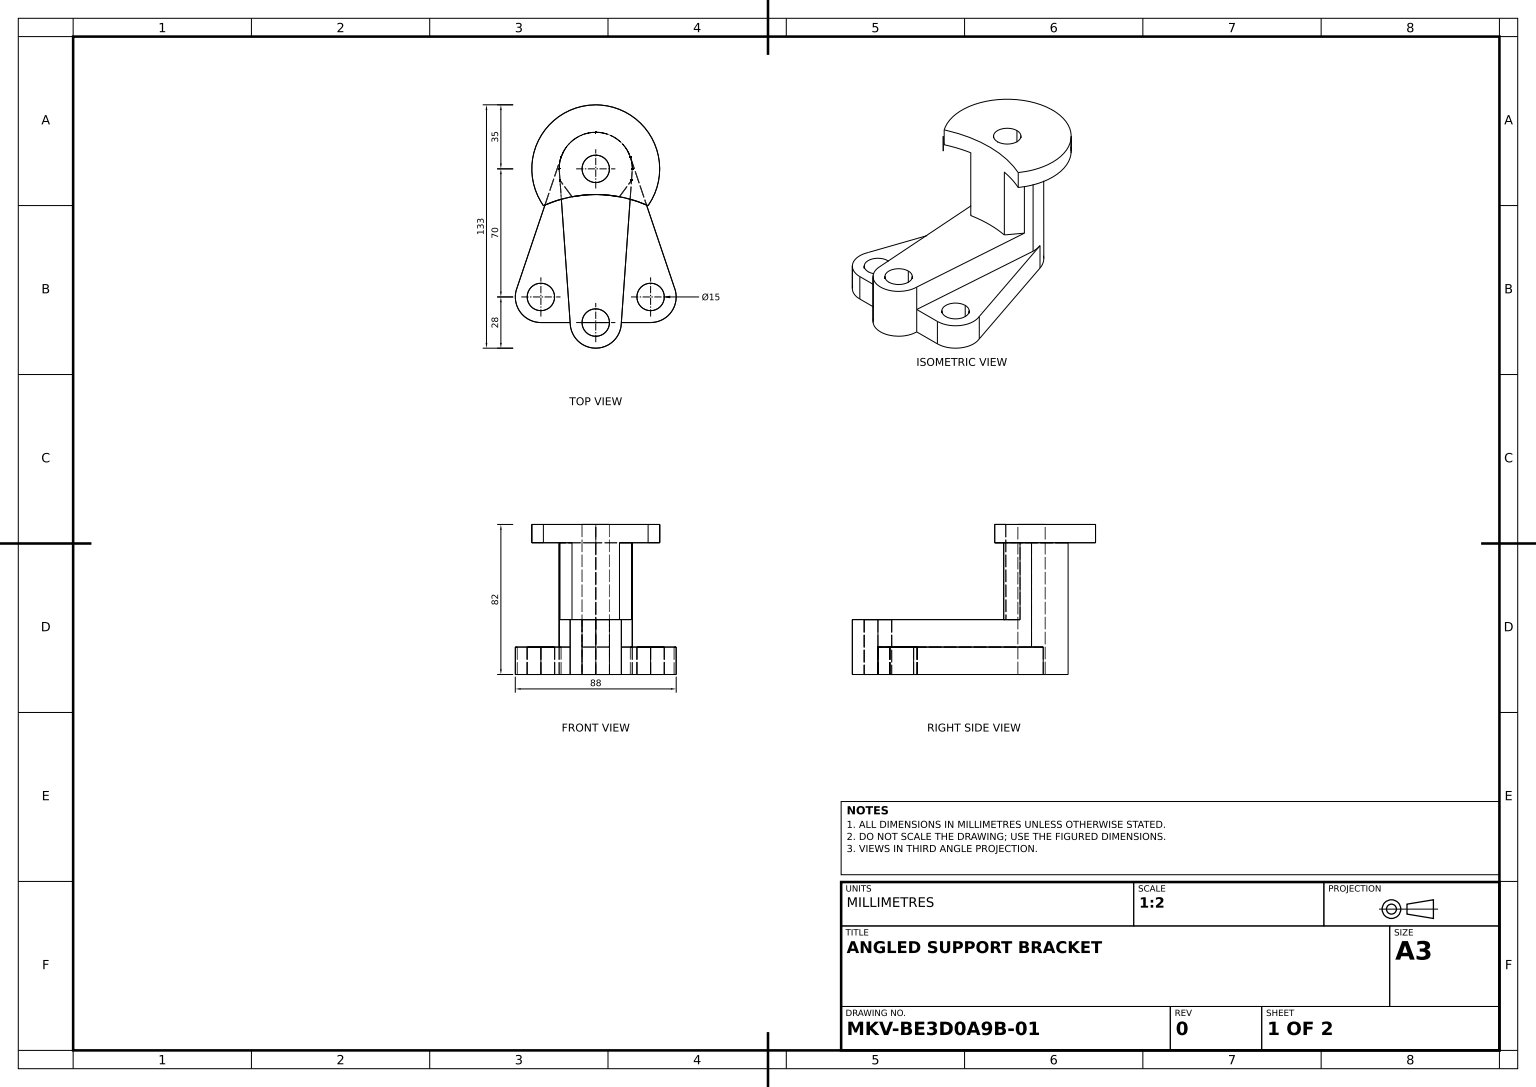
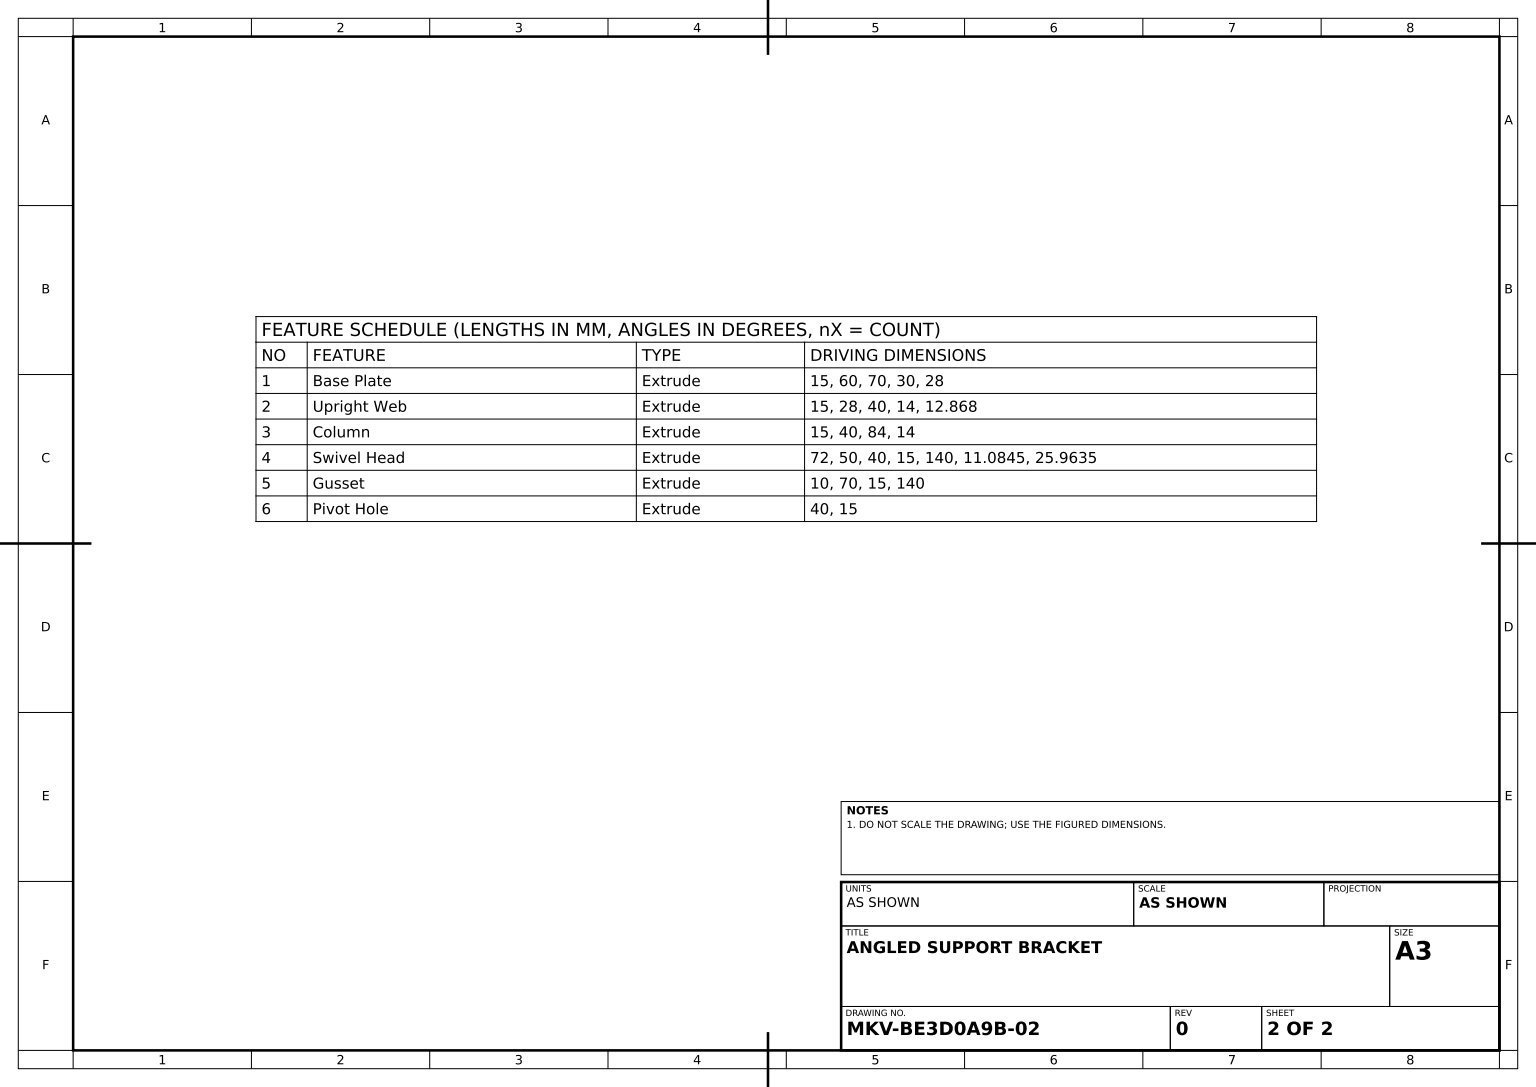
from build123d import *

# Parameters (mm, degrees)
BASE_PLATE_SKETCH_R  = 7.5
BASE_PLATE_DEPTH     = 15
UPRIGHT_WEB_SKETCH_R = 7.5
UPRIGHT_WEB_DEPTH    = 15
COLUMN_DEPTH         = 15
SWIVEL_START         = -50
SWIVEL_HEAD_SKETCH_R = 7.5
SWIVEL_HEAD_DEPTH    = 50
GUSSET_SKETCH_R      = 7.5
GUSSET_DEPTH         = 10
PIVOT_START          = -40
PIVOT_HOLE_SKETCH_R  = 7.5
PIVOT_HOLE_DEPTH     = 40


with BuildPart() as part:
    # Base Plate Sketch → Base Plate (new body)
    with BuildSketch(Plane(origin=(0, 0, 0), x_dir=(1, 0, 0), z_dir=(0, 1, 0))):
        with BuildLine():
            Line((17.13196958, 75.51487018), (-12.86803042, 5.51487018))
            ThreePointArc((-12.86803042, 5.51487018), (-11.687775291, -7.706874122), (0, -14))
            Line((0, -14), (60, -14))
            ThreePointArc((60, -14), (71.687775291, -7.706874122), (72.86803042, 5.51487018))
            Line((72.86803042, 5.51487018), (42.86803042, 75.51487018))
            ThreePointArc((42.86803042, 75.51487018), (30, 84), (17.13196958, 75.51487018))
        make_face()
        with Locations(Location((0, 0, 0), (0, 0, 270))):
            Circle(BASE_PLATE_SKETCH_R, mode=Mode.SUBTRACT)
        with Locations(Location((60, 0, 0), (0, 0, 270))):
            Circle(BASE_PLATE_SKETCH_R, mode=Mode.SUBTRACT)
        with Locations(Location((30, 70, 0), (0, 0, 270))):
            Circle(BASE_PLATE_SKETCH_R, mode=Mode.SUBTRACT)
    extrude(amount=BASE_PLATE_DEPTH)

    # Upright Web Sketch → Upright Web (add)
    with BuildSketch(Plane.XZ):
        with BuildLine():
            Line((-12.86803042, -5.51487018), (11.049826186, -76.394600254))
            ThreePointArc((11.049826186, -76.394600254), (30, -90), (48.950173814, -76.394600254))
            Line((48.950173814, -76.394600254), (72.86803042, -5.51487018))
            ThreePointArc((72.86803042, -5.51487018), (71.687775291, 7.706874122), (60, 14))
            Line((60, 14), (44, 14))
            ThreePointArc((44, 14), (30, 28), (16, 14))
            Line((16, 14), (0, 14))
            ThreePointArc((0, 14), (-11.687775291, 7.706874122), (-12.86803042, -5.51487018))
        make_face()
        with Locations((30, 14)):
            Circle(UPRIGHT_WEB_SKETCH_R, mode=Mode.SUBTRACT)
        with Locations(Location((0, 0, 0), (0, 0, 90))):
            Circle(UPRIGHT_WEB_SKETCH_R, mode=Mode.SUBTRACT)
        with Locations(Location((60, 0, 0), (0, 0, 90))):
            Circle(UPRIGHT_WEB_SKETCH_R, mode=Mode.SUBTRACT)
    extrude(amount=-UPRIGHT_WEB_DEPTH)

    # Column Sketch → Column (add)
    with BuildSketch(Plane(origin=(0, 15, 0), x_dir=(1, 0, 0), z_dir=(0, 1, 0))):
        with BuildLine():
            ThreePointArc((11.049826186, 76.394600254), (10.264201609, 73.240102137), (10, 70))
            Line((10, 70), (10.203045685, 67.157360406))
            Line((10.203045685, 67.157360406), (16, -14))
            ThreePointArc((16, -14), (30, -28), (44, -14))
            Line((44, -14), (49.796954315, 67.157360406))
            Line((49.796954315, 67.157360406), (50, 70))
            ThreePointArc((50, 70), (49.735798391, 73.240102137), (48.950173814, 76.394600254))
            ThreePointArc((48.950173814, 76.394600254), (30, 90), (11.049826186, 76.394600254))
        make_face()
        with BuildLine():
            ThreePointArc((37.5, -14), (30, -21.5), (22.5, -14))
            ThreePointArc((22.5, -14), (30, -6.5), (37.5, -14))
        make_face(mode=Mode.SUBTRACT)
    extrude(amount=COLUMN_DEPTH)

    # Swivel Head Sketch → Swivel Head (add)
    with BuildSketch(Plane(origin=(0, 72, 0), x_dir=(1, 0, 0), z_dir=(0, 1, 0)).offset(SWIVEL_START)):
        with BuildLine():
            ThreePointArc((17.018262435, 54.785714286), (30, 56), (42.981737565, 54.785714286))
            Line((42.981737565, 54.785714286), (49.550987537, 63.713825524))
            Line((49.550987537, 63.713825524), (49.796954315, 67.157360406))
            Line((49.796954315, 67.157360406), (50, 70))
            ThreePointArc((50, 70), (30, 90), (10, 70))
            Line((10, 70), (10.203045685, 67.157360406))
            Line((10.203045685, 67.157360406), (10.449012463, 63.713825524))
            Line((10.449012463, 63.713825524), (17.018262435, 54.785714286))
        make_face()
        with Locations(Location((30, 70, 0), (0, 0, 270))):
            Circle(SWIVEL_HEAD_SKETCH_R, mode=Mode.SUBTRACT)
    extrude(amount=SWIVEL_HEAD_DEPTH)

    # Gusset Sketch → Gusset (add)
    with BuildSketch(Plane(origin=(0, 72, 0), x_dir=(1, 0, 0), z_dir=(0, 1, 0))):
        with BuildLine():
            ThreePointArc((58.635369301, 49.875), (30, 105), (1.364630699, 49.875))
            ThreePointArc((1.364630699, 49.875), (30, 56), (58.635369301, 49.875))
        make_face()
        with Locations(Location((30, 70, 0), (0, 0, 270))):
            Circle(GUSSET_SKETCH_R, mode=Mode.SUBTRACT)
    extrude(amount=GUSSET_DEPTH)

    # Pivot Hole Sketch → Pivot Hole (cut)
    with BuildSketch(Plane(origin=(0, 30, 0), x_dir=(1, 0, 0), z_dir=(0, 1, 0)).offset(PIVOT_START)):
        with Locations(Location((30, 70, 0), (0, 0, 270))):
            Circle(PIVOT_HOLE_SKETCH_R)
    extrude(amount=PIVOT_HOLE_DEPTH, mode=Mode.SUBTRACT)


solid = part.part
